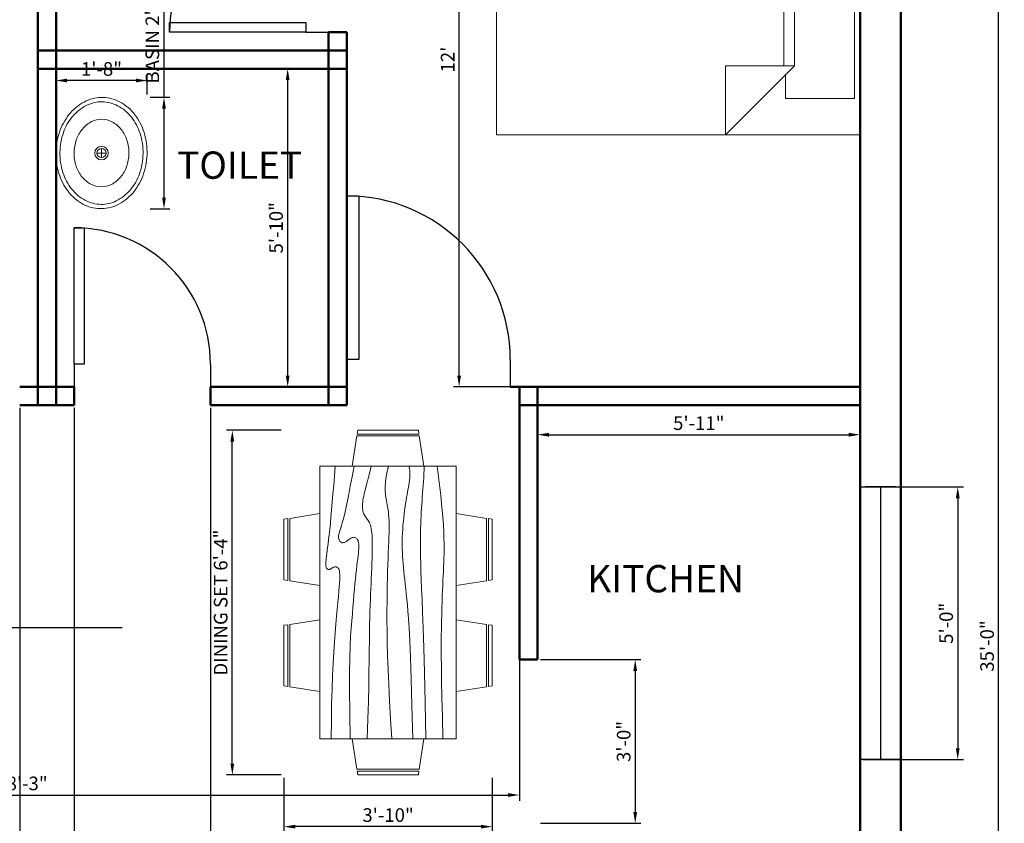
# Model space of a CAD drawing. Units: inches. Extents: x 1767 to 2185, y 3382 to 3854.
# Tile 3 of 4: x 1950 to 2167, y 3577 to 3754. Entities that reach past the tile are written whole.
import ezdxf

# ---------------------------------------------------------------- set-up
doc = ezdxf.new("R2010")
doc.units = ezdxf.units.IN
for name, color, linetype, lineweight in [('A-ANNO-DIMS', 2, 'Continuous', 18), ('A-AREA-IDEN', 7, 'Continuous', 25), ('A-DOOR', 3, 'Continuous', 25), ('A-FLOR-FIXT', 9, 'Continuous', 20), ('A-FURN', 8, 'Continuous', 18), ('A-GLAZ', 4, 'Continuous', 25), ('A-WALL', 7, 'Continuous', 50)]:
    doc.layers.add(name, color=color, linetype=linetype, lineweight=lineweight)
doc.styles.get("Standard").update_dxf_attribs({"font": 'arial.ttf'})
doc.dimstyles.new('ISO-25', dxfattribs={"dimtxt": 3, "dimasz": 2.5, "dimexe": 1.25, "dimexo": 0.625, "dimtad": 1, "dimdec": 0, "dimlunit": 3, "dimtxsty": 'Standard', "dimcen": 2.5, "dimadec": 0, "dimazin": 0, "dimtfac": 1, "dimtdec": 0, "dimtmove": 0, "dimatfit": 3, "dimfxl": 1, "dimarcsym": 0})

# ---------------------------------------------------------------- blocks, each defined once
blk = doc.blocks.new('*U2')
for p, q in [((0, 0), (0, -100)), ((600, 0), (600, -100))]:
    blk.add_line(p, q)
blk.add_lwpolyline([(0, 0), (0, 600), (43.75, 600), (43.75, 0)], close=True)
blk.add_arc((0, 0), 600, 0, 90)
blk = doc.blocks.new('*U4')
for p, q in [((0, 100), (0, 0)), ((900, 100), (900, 0)), ((0, 50), (900, 50))]:
    blk.add_line(p, q)
blk = doc.blocks.new('Dining Set - 36 x 72 in.')
for p, q in [((-22, 27.5), (-22.1562, 26.50042)), ((-5.8416, 26.5), (-22.1534, 26.5)), ((-22, 27.5), (-6, 27.5)), ((-5.8437, 26.49966), (-6, 27.5)), ((6, 27.5), (5.8438, 26.50042)), ((22.1584, 26.5), (5.8466, 26.5)), ((6, 27.5), (22, 27.5)), ((22.1563, 26.49966), (22, 27.5)), ((-22.2343, 26.00059), (-23.4847, 17.99762)), ((-22.2304, 26), (-5.7608, 26)), ((-4.5152, 17.99762), (-5.7655, 25.99926)), ((5.7657, 26.00059), (4.5153, 17.99762)), ((5.7696, 26), (22.2392, 26)), ((23.4848, 17.99762), (22.2345, 25.99926)), ((36, 18), (-36, 18)), ((-36, 18), (-36, -18)), ((36, -18), (36, 18)), ((-45.5, 8), (-44.5004, 8.15617)), ((-45.5, 8), (-45.5, -8)), ((-44.5, -8.15843), (-44.5, 8.15338)), ((-44.0006, 8.23428), (-35.9976, 9.48474)), ((-44, 8.23041), (-44, -8.23915)), ((44.0006, 8.23428), (35.9976, 9.48474)), ((44, 8.23041), (44, -8.23915)), ((44.5, -8.15843), (44.5, 8.15338)), ((45.5, 8), (44.5005, 8.15617)), ((45.5, 8), (45.5, -8)), ((-44.4997, -8.15631), (-45.5, -8)), ((-35.9976, -9.48476), (-43.9993, -8.2345)), ((35.9976, -9.48476), (43.9993, -8.2345)), ((44.4997, -8.15631), (45.5, -8)), ((-36, -18), (36, -18)), ((-22.2343, -26.0006), (-23.4847, -17.99762)), ((-4.5152, -17.99762), (-5.7655, -25.99928)), ((5.7657, -26.0006), (4.5153, -17.99762)), ((23.4848, -17.99762), (22.2345, -25.99928)), ((-22.2304, -26), (-5.7608, -26)), ((5.7696, -26), (22.2392, -26)), ((-22, -27.5), (-22.1562, -26.50044)), ((-5.8416, -26.5), (-22.1534, -26.5)), ((-22, -27.5), (-6, -27.5)), ((-5.8437, -26.49967), (-6, -27.5)), ((6, -27.5), (5.8438, -26.50044)), ((22.1584, -26.5), (5.8466, -26.5)), ((6, -27.5), (22, -27.5)), ((22.1563, -26.49967), (22, -27.5))]:
    blk.add_line(p, q)
for points in [[(-36, 15), (-31.1772, 14.97754), (-26.8079, 14.91406), (-22.8538, 14.81543), (-19.276, 14.6875), (-16.0362, 14.53613), (-13.0957, 14.36718), (-10.4159, 14.18652), (-7.9583, 14), (-5.6904, 13.81315), (-3.6035, 13.63021), (-1.6954, 13.45508), (0.0365, 13.29166), (1.5945, 13.14388), (2.9811, 13.01562), (4.1988, 12.9108), (5.25, 12.83333), (6.1393, 12.78613), (6.8802, 12.76823), (7.4883, 12.77767), (7.9792, 12.8125), (8.3685, 12.87077), (8.6719, 12.95052), (8.9049, 13.0498), (9.0833, 13.16666), (9.2205, 13.29899), (9.3216, 13.44401), (9.3895, 13.59879), (9.4271, 13.76041), (9.4373, 13.92594), (9.4232, 14.09245), (9.3875, 14.257), (9.3333, 14.41666), (9.2638, 14.56917), (9.1836, 14.71484), (9.0975, 14.85465), (9.0104, 14.98958), (8.9272, 15.1206), (8.8529, 15.2487), (8.7922, 15.37483), (8.75, 15.5), (8.7305, 15.62467), (8.7344, 15.74739), (8.7617, 15.86621), (8.8125, 15.97916), (8.8867, 16.08431), (8.9844, 16.17968), (9.1055, 16.26334), (9.25, 16.33333), (9.4189, 16.38802), (9.6172, 16.42708), (9.8506, 16.45052), (10.125, 16.45833), (10.4463, 16.45052), (10.8203, 16.42708), (11.2529, 16.38802), (11.75, 16.33333), (12.3184, 16.26318), (12.9694, 16.17838), (13.7151, 16.07991), (14.5677, 15.96875), (15.5395, 15.84586), (16.6426, 15.71224), (17.8893, 15.56884), (19.2917, 15.41666), (20.859, 15.25667), (22.5879, 15.08984), (24.4721, 14.91715), (26.5052, 14.73958), (28.6809, 14.5581), (30.9929, 14.3737), (33.4347, 14.18733), (36, 14)], [(-36, 10), (-28.9766, 10.14274), (-23.1725, 10.20442), (-18.4241, 10.19775), (-14.5677, 10.13541), (-11.4399, 10.03011), (-8.877, 9.89453), (-6.7154, 9.74137), (-4.7917, 9.58333), (-2.9698, 9.43082), (-1.2246, 9.28515), (0.4415, 9.14534), (2.026, 9.01041), (3.5266, 8.87939), (4.9408, 8.7513), (6.266, 8.62516), (7.5, 8.5), (8.6411, 8.37549), (9.6914, 8.2539), (10.6538, 8.13818), (11.5312, 8.03125), (12.3267, 7.93603), (13.043, 7.85547), (13.6831, 7.79248), (14.25, 7.75), (14.7471, 7.7303), (15.1797, 7.73307), (15.5537, 7.75732), (15.875, 7.80208), (16.1494, 7.86637), (16.3828, 7.94922), (16.5811, 8.04964), (16.75, 8.16666), (16.8944, 8.29915), (17.0143, 8.44531), (17.1089, 8.60319), (17.1771, 8.77083), (17.218, 8.94629), (17.2305, 9.1276), (17.2137, 9.31282), (17.1667, 9.5), (17.0895, 9.6875), (16.987, 9.875), (16.8649, 10.0625), (16.7292, 10.25), (16.5856, 10.4375), (16.4401, 10.625), (16.2985, 10.8125), (16.1667, 11), (16.05, 11.18733), (15.9518, 11.3737), (15.8752, 11.5581), (15.8229, 11.73958), (15.798, 11.91715), (15.8034, 12.08984), (15.842, 12.25667), (15.9167, 12.41666), (16.0295, 12.56836), (16.1784, 12.70833), (16.3605, 12.83268), (16.5729, 12.9375), (16.8127, 13.01888), (17.0768, 13.07291), (17.3625, 13.0957), (17.6667, 13.08333), (17.9894, 13.03312), (18.3418, 12.94726), (18.7382, 12.82918), (19.1927, 12.68229), (19.7195, 12.51001), (20.3327, 12.31575), (21.0465, 12.10294), (21.875, 11.875), (22.8357, 11.63354), (23.959, 11.37304), (25.2786, 11.08618), (26.8282, 10.76562), (28.6414, 10.40405), (30.752, 9.99414), (33.1936, 9.52856), (36, 9)], [(-36, 5.5), (-30.7157, 5.3348), (-26.069, 5.20963), (-21.9946, 5.11767), (-18.4271, 5.05208), (-15.3009, 5.00602), (-12.5508, 4.97265), (-10.1112, 4.94515), (-7.9167, 4.91666), (-5.909, 4.88167), (-4.0586, 4.83984), (-2.3429, 4.79215), (-0.7396, 4.73958), (0.7739, 4.6831), (2.22, 4.6237), (3.6213, 4.56233), (5, 4.5), (6.373, 4.43782), (7.7344, 4.3776), (9.0723, 4.32129), (10.375, 4.27083), (11.6309, 4.22819), (12.8281, 4.19531), (13.9551, 4.17415), (15, 4.16666), (15.954, 4.17448), (16.819, 4.19791), (17.6001, 4.23698), (18.3021, 4.29166), (18.9299, 4.36198), (19.4883, 4.44791), (19.9823, 4.54948), (20.4167, 4.66666), (20.7969, 4.79899), (21.1302, 4.94401), (21.4245, 5.09879), (21.6875, 5.26041), (21.9271, 5.42594), (22.1511, 5.59245), (22.3672, 5.757), (22.5834, 5.91666), (22.8065, 6.06868), (23.0404, 6.21093), (23.2879, 6.34147), (23.5521, 6.45833), (23.8358, 6.55957), (24.142, 6.64323), (24.4735, 6.70735), (24.8334, 6.75), (25.2235, 6.76969), (25.642, 6.76692), (26.0858, 6.74267), (26.5521, 6.69791), (27.0379, 6.63362), (27.5404, 6.55078), (28.0565, 6.45036), (28.5834, 6.33333), (29.1242, 6.19987), (29.7071, 6.04687), (30.3661, 5.87044), (31.1354, 5.66666), (32.0493, 5.43164), (33.142, 5.16146), (34.4475, 4.85221), (36, 4.5)], [(-36, -1), (-30.7915, -0.6591), (-26.0195, -0.38216), (-21.6519, -0.16284), (-17.6563, 0.00521), (-14.0005, 0.12833), (-10.6523, 0.21289), (-7.5796, 0.26522), (-4.75, 0.29166), (-2.134, 0.29793), (0.2878, 0.28711), (2.5317, 0.26163), (4.6146, 0.22396), (6.5529, 0.17651), (8.3633, 0.12174), (10.0623, 0.06209), (11.6667, 0), (13.1899, -0.06201), (14.6341, -0.1211), (15.9982, -0.17432), (17.2813, -0.21875), (18.4823, -0.25147), (19.6003, -0.26953), (20.6343, -0.27002), (21.5834, -0.25), (22.4481, -0.20768), (23.2357, -0.14584), (23.9549, -0.06836), (24.6146, 0.02083), (25.2235, 0.11784), (25.7904, 0.21875), (26.3241, 0.31966), (26.8334, 0.41666), (27.3265, 0.50618), (27.8099, 0.58593), (28.2894, 0.65397), (28.7709, 0.70833), (29.2601, 0.74707), (29.763, 0.76823), (30.2855, 0.76985), (30.8334, 0.75), (31.4088, 0.70784), (31.9994, 0.64713), (32.589, 0.57275), (33.1615, 0.48958), (33.7008, 0.4025), (34.1908, 0.3164), (34.6153, 0.23616), (34.9584, 0.16666), (35.2099, 0.11165), (35.3848, 0.07031), (35.504, 0.04069), (35.5886, 0.02083), (35.6594, 0.00879), (35.7377, 0.0026), (35.8442, 0.00032), (36, 0)], [(-36, -6.5), (-27.1843, -6.31267), (-20.084, -6.1263), (-14.469, -5.9419), (-10.1094, -5.76042), (-6.7752, -5.58285), (-4.2363, -5.41016), (-2.2629, -5.24333), (-0.625, -5.08334), (0.8708, -4.93099), (2.2715, -4.78646), (3.5872, -4.64974), (4.8281, -4.52084), (6.0046, -4.39974), (7.127, -4.28646), (8.2053, -4.18099), (9.25, -4.08334), (10.2705, -3.99382), (11.2734, -3.91407), (12.2647, -3.84603), (13.25, -3.79167), (14.2354, -3.75293), (15.2266, -3.73177), (16.2295, -3.73015), (17.25, -3.75), (18.2912, -3.79248), (19.3451, -3.85547), (20.4009, -3.93604), (21.4479, -4.03125), (22.4754, -4.13819), (23.4727, -4.25391), (24.4289, -4.37549), (25.3334, -4.5), (26.1785, -4.62492), (26.9694, -4.74935), (27.7145, -4.87281), (28.4219, -4.99479), (29.1, -5.11483), (29.7572, -5.23242), (30.4016, -5.34709), (31.0417, -5.45834), (31.6837, -5.56437), (32.3262, -5.65821), (32.9658, -5.73153), (33.599, -5.77604), (34.2224, -5.78345), (34.8327, -5.74545), (35.4264, -5.65373), (36, -5.5)], [(-36, -10), (-26.4022, -9.81299), (-18.4675, -9.62891), (-11.9839, -9.45069), (-6.7396, -9.28125), (-2.5226, -9.12354), (0.8789, -8.98047), (3.6769, -8.85498), (6.0833, -8.75), (8.2767, -8.66765), (10.3021, -8.60677), (12.1712, -8.56543), (13.8958, -8.54167), (15.4876, -8.53353), (16.9583, -8.53907), (18.3197, -8.55632), (19.5834, -8.58334), (20.7616, -8.61841), (21.8685, -8.66081), (22.9188, -8.71004), (23.9271, -8.76563), (24.9081, -8.82707), (25.8763, -8.89388), (26.8465, -8.96558), (27.8334, -9.04167), (28.8474, -9.12118), (29.8828, -9.20117), (30.93, -9.27824), (31.9792, -9.34896), (33.0205, -9.40991), (34.0443, -9.45768), (35.0407, -9.48885), (36, -9.5)], [(-36, -14.5), (-30.0881, -14.33513), (-25.0332, -14.21224), (-20.7312, -14.12647), (-17.0781, -14.07292), (-13.97, -14.04671), (-11.3027, -14.04297), (-8.9724, -14.05681), (-6.875, -14.08334), (-4.9224, -14.11833), (-3.0905, -14.16016), (-1.3709, -14.20785), (0.2448, -14.26042), (1.7647, -14.3169), (3.1973, -14.3763), (4.5507, -14.43767), (5.8333, -14.5), (7.0554, -14.5621), (8.235, -14.62175), (9.3922, -14.67652), (10.5469, -14.72396), (11.7192, -14.76164), (12.929, -14.78711), (14.1965, -14.79794), (15.5417, -14.79167), (16.9933, -14.76424), (18.6152, -14.70508), (20.4804, -14.60197), (22.6615, -14.44271), (25.2312, -14.21509), (28.2624, -13.9069), (31.8277, -13.50594), (36, -13)]]:
    blk.add_lwpolyline(points)
blk = doc.blocks.new('Sink - Oval top')
for p, q in [((-1, 0), (1, 0)), ((0, 1), (0, -1))]:
    blk.add_line(p, q)
for points in [[(-12.23, 0.39, 0.117634), (-11.46, -3.36, 0.104469), (-8.88, -6.8, 0.090016), (-5.08, -9.07, 0.08192), (-0.32, -10.02, 0.08192), (4.49, -9.38, 0.090016), (8.42, -7.36, 0.104469), (11.22, -4.09, 0.117634), (12.23, -0.39, 0.117634), (11.46, 3.36, 0.104469), (8.88, 6.8, 0.090016), (5.08, 9.07, 0.08192), (0.32, 10.02, 0.08192), (-4.49, 9.38, 0.090016), (-8.42, 7.36, 0.104469), (-11.22, 4.09, 0.117634)], [(-11.29, 0.16, 0.118622), (-10.52, -3.25, 0.104678), (-8.07, -6.36, 0.089562), (-4.54, -8.37, 0.081185), (-0.13, -9.15, 0.081185), (4.3, -8.49, 0.089562), (7.89, -6.58, 0.104678), (10.42, -3.55, 0.118622), (11.29, -0.16, 0.118622), (10.52, 3.25, 0.104678), (8.07, 6.36, 0.089562), (4.54, 8.37, 0.081185), (0.13, 9.15, 0.081185), (-4.3, 8.49, 0.089562), (-7.89, 6.58, 0.104678), (-10.42, 3.55, 0.118622)], [(-7.42, 0.08, 0.118283), (-6.91, -2.17, 0.104607), (-5.29, -4.21, 0.089718), (-2.97, -5.53, 0.081436), (-0.07, -6.04, 0.081436), (2.84, -5.59, 0.089718), (5.2, -4.33, 0.104607), (6.86, -2.32, 0.118283), (7.42, -0.08, 0.118283), (6.91, 2.17, 0.104607), (5.29, 4.21, 0.089718), (2.97, 5.53, 0.081436), (0.07, 6.04, 0.081436), (-2.84, 5.59, 0.089718), (-5.2, 4.33, 0.104607), (-6.86, 2.32, 0.118283)]]:
    blk.add_lwpolyline(points, format="xyb", close=True)
for radius in [1.5, 1]:
    blk.add_circle((0, 0), radius)
blk = doc.blocks.new('Bed - Queen')
for p, q in [((0, -80.00003), (0, 0)), ((0, 0), (59.99999, 0)), ((59.99999, 0), (59.99999, -80.00003)), ((7.99999, -1.2), (28.79998, -1.2)), ((7.99999, -14.4), (7.99999, -1.2)), ((28.79998, -1.2), (28.79998, -14.4)), ((31.19999, -1.2), (51.99999, -1.2)), ((31.19999, -14.4), (31.19999, -1.2)), ((51.99999, -1.2), (51.99999, -16.4)), ((0, -14.4), (44.8, -14.4)), ((59.99999, -29.6), (44.8, -14.4)), ((44.8, -14.4), (44.8, -29.6)), ((44.8, -16.8), (0, -16.8)), ((51.99999, -16.4), (46.79936, -16.4)), ((44.8, -29.6), (59.99999, -29.6)), ((59.99999, -80.00003), (0, -80.00003))]:
    blk.add_line(p, q)
blk = doc.blocks.new('*D13')
at = {"layer": 'A-ANNO-DIMS', "color": 0, "lineweight": -2, "transparency": 16777216}
for p, q in [((2134.53, 3817.15), (2045.65, 3817.15)), ((2046.9, 3675.65), (2046.9, 3814.65)), ((2134.53, 3673.15), (2045.65, 3673.15))]:
    blk.add_line(p, q, dxfattribs=at)
at = {"layer": 'A-ANNO-DIMS', "color": 0, "transparency": 16777216}
for points in [[(2046.48, 3814.65), (2047.32, 3814.65), (2046.9, 3817.15)], [(2046.48, 3675.65), (2047.32, 3675.65), (2046.9, 3673.15)]]:
    blk.add_solid(points, dxfattribs=at)
at = {"layer": 'Defpoints', "color": 0, "transparency": 16777216}
for p in [(2046.9, 3817.15), (2135.16, 3817.15), (2135.16, 3673.15)]:
    blk.add_point(p, dxfattribs=at)
at = {"layer": 'A-ANNO-DIMS', "color": 0, "transparency": 16777216, "insert": (2044.77, 3745.15), "char_height": 3, "attachment_point": 5, "rotation": 90}
blk.add_mtext("12'", dxfattribs=at)
blk = doc.blocks.new('*D15')
at = {"layer": 'A-ANNO-DIMS', "color": 0, "lineweight": -2, "transparency": 16777216}
for p, q in [((2017.53, 3743.15), (2007.9, 3743.15)), ((2009.15, 3740.65), (2009.15, 3675.65)), ((2017.53, 3673.15), (2007.9, 3673.15))]:
    blk.add_line(p, q, dxfattribs=at)
at = {"layer": 'A-ANNO-DIMS', "color": 0, "transparency": 16777216}
for points in [[(2008.73, 3740.65), (2009.57, 3740.65), (2009.15, 3743.15)], [(2008.73, 3675.65), (2009.57, 3675.65), (2009.15, 3673.15)]]:
    blk.add_solid(points, dxfattribs=at)
at = {"layer": 'Defpoints', "color": 0, "transparency": 16777216}
for p in [(2018.16, 3743.15), (2009.15, 3673.15), (2018.16, 3673.15)]:
    blk.add_point(p, dxfattribs=at)
at = {"layer": 'A-ANNO-DIMS', "color": 0, "transparency": 16777216, "insert": (2006.99, 3708.15), "char_height": 3, "attachment_point": 5, "rotation": 90}
blk.add_mtext('5\'-10"', dxfattribs=at)
blk = doc.blocks.new('*D16')
at = {"layer": 'A-ANNO-DIMS', "color": 0, "lineweight": -2, "transparency": 16777216}
for p, q in [((2064.16, 3668.53), (2064.16, 3661.38)), ((2135.16, 3668.53), (2135.16, 3661.38)), ((2066.66, 3662.63), (2132.66, 3662.63))]:
    blk.add_line(p, q, dxfattribs=at)
at = {"layer": 'A-ANNO-DIMS', "color": 0, "transparency": 16777216}
for points in [[(2066.66, 3663.04), (2066.66, 3662.21), (2064.16, 3662.63)], [(2132.66, 3663.04), (2132.66, 3662.21), (2135.16, 3662.63)]]:
    blk.add_solid(points, dxfattribs=at)
at = {"layer": 'Defpoints', "color": 0, "transparency": 16777216}
for p in [(2064.16, 3669.15), (2135.16, 3669.15), (2135.16, 3662.63)]:
    blk.add_point(p, dxfattribs=at)
at = {"layer": 'A-ANNO-DIMS', "color": 0, "transparency": 16777216, "insert": (2099.66, 3664.78), "char_height": 3, "attachment_point": 5}
blk.add_mtext('5\'-11"', dxfattribs=at)
blk = doc.blocks.new('*D17')
at = {"layer": 'A-ANNO-DIMS', "color": 0, "lineweight": -2, "transparency": 16777216}
for p, q in [((1841.16, 3668.53), (1841.16, 3582.12)), ((2060.16, 3668.53), (2060.16, 3582.12)), ((1843.66, 3583.37), (2057.66, 3583.37))]:
    blk.add_line(p, q, dxfattribs=at)
at = {"layer": 'A-ANNO-DIMS', "color": 0, "transparency": 16777216}
for points in [[(1843.66, 3583.79), (1843.66, 3582.96), (1841.16, 3583.37)], [(2057.66, 3583.79), (2057.66, 3582.96), (2060.16, 3583.37)]]:
    blk.add_solid(points, dxfattribs=at)
at = {"layer": 'Defpoints', "color": 0, "transparency": 16777216}
for p in [(1841.16, 3669.15), (2060.16, 3669.15), (2060.16, 3583.37)]:
    blk.add_point(p, dxfattribs=at)
at = {"layer": 'A-ANNO-DIMS', "color": 0, "transparency": 16777216, "insert": (1950.66, 3585.53), "char_height": 3, "attachment_point": 5}
blk.add_mtext('18\'-3"', dxfattribs=at)
blk = doc.blocks.new('*D31')
at = {"layer": 'A-ANNO-DIMS', "color": 0, "lineweight": -2, "transparency": 16777216}
for p, q in [((2007.72, 3663.62), (1995.72, 3663.62)), ((1996.97, 3590.29), (1996.97, 3661.12)), ((2007.72, 3587.79), (1995.72, 3587.79))]:
    blk.add_line(p, q, dxfattribs=at)
at = {"layer": 'A-ANNO-DIMS', "color": 0, "transparency": 16777216}
for points in [[(1996.55, 3661.12), (1997.38, 3661.12), (1996.97, 3663.62)], [(1996.55, 3590.29), (1997.38, 3590.29), (1996.97, 3587.79)]]:
    blk.add_solid(points, dxfattribs=at)
at = {"layer": 'Defpoints', "color": 0, "transparency": 16777216}
for p in [(1996.97, 3663.62), (2008.34, 3663.62), (2008.34, 3587.79)]:
    blk.add_point(p, dxfattribs=at)
at = {"layer": 'A-ANNO-DIMS', "color": 0, "transparency": 16777216, "insert": (1994.79, 3625.7), "char_height": 3, "attachment_point": 5, "rotation": 90}
blk.add_mtext('DINING SET 6\'-4"', dxfattribs=at)
blk = doc.blocks.new('*D32')
at = {"layer": 'A-ANNO-DIMS', "color": 0, "lineweight": -2, "transparency": 16777216}
for p, q in [((2008.34, 3587.16), (2008.34, 3575.16)), ((2054.18, 3587.16), (2054.18, 3575.16)), ((2051.68, 3576.41), (2010.84, 3576.41))]:
    blk.add_line(p, q, dxfattribs=at)
at = {"layer": 'A-ANNO-DIMS', "color": 0, "transparency": 16777216}
for points in [[(2010.84, 3576.83), (2010.84, 3576), (2008.34, 3576.41)], [(2051.68, 3576.83), (2051.68, 3576), (2054.18, 3576.41)]]:
    blk.add_solid(points, dxfattribs=at)
at = {"layer": 'Defpoints', "color": 0, "transparency": 16777216}
for p in [(2008.34, 3587.79), (2054.18, 3587.79), (2008.34, 3576.41)]:
    blk.add_point(p, dxfattribs=at)
at = {"layer": 'A-ANNO-DIMS', "color": 0, "transparency": 16777216, "insert": (2031.26, 3578.57), "char_height": 3, "attachment_point": 5}
blk.add_mtext('3\'-10"', dxfattribs=at)
blk = doc.blocks.new('*D35')
at = {"layer": 'A-ANNO-DIMS', "color": 0, "lineweight": -2, "transparency": 16777216}
for p, q in [((1981.93, 3736.86), (1981.93, 3769.19)), ((1978.87, 3736.86), (1983.18, 3736.86)), ((1981.93, 3714.81), (1981.93, 3734.36)), ((1978.87, 3712.31), (1983.18, 3712.31))]:
    blk.add_line(p, q, dxfattribs=at)
at = {"layer": 'A-ANNO-DIMS', "color": 0, "transparency": 16777216}
for points in [[(1981.51, 3734.36), (1982.34, 3734.36), (1981.93, 3736.86)], [(1981.51, 3714.81), (1982.34, 3714.81), (1981.93, 3712.31)]]:
    blk.add_solid(points, dxfattribs=at)
at = {"layer": 'Defpoints', "color": 0, "transparency": 16777216}
for p in [(1978.24, 3736.86), (1981.93, 3736.86), (1978.24, 3712.31)]:
    blk.add_point(p, dxfattribs=at)
at = {"layer": 'A-ANNO-DIMS', "color": 0, "transparency": 16777216, "insert": (1979.75, 3754.28), "char_height": 3, "attachment_point": 5, "rotation": 90}
blk.add_mtext('BASIN 2\'-0 1/2"', dxfattribs=at)
blk = doc.blocks.new('*D36')
at = {"layer": 'A-ANNO-DIMS', "color": 0, "lineweight": -2, "transparency": 16777216}
for p, q in [((1958.11, 3737.49), (1958.11, 3741.8)), ((1978.24, 3737.49), (1978.24, 3741.8)), ((1975.74, 3740.55), (1960.61, 3740.55))]:
    blk.add_line(p, q, dxfattribs=at)
at = {"layer": 'A-ANNO-DIMS', "color": 0, "transparency": 16777216}
for points in [[(1960.61, 3740.96), (1960.61, 3740.13), (1958.11, 3740.55)], [(1975.74, 3740.96), (1975.74, 3740.13), (1978.24, 3740.55)]]:
    blk.add_solid(points, dxfattribs=at)
at = {"layer": 'Defpoints', "color": 0, "transparency": 16777216}
for p in [(1958.11, 3740.55), (1958.11, 3736.86), (1978.24, 3736.86)]:
    blk.add_point(p, dxfattribs=at)
at = {"layer": 'A-ANNO-DIMS', "color": 0, "transparency": 16777216, "insert": (1968.17, 3742.7), "char_height": 3, "attachment_point": 5}
blk.add_mtext('1\'-8"', dxfattribs=at)
blk = doc.blocks.new('*D40')
at = {"layer": 'A-ANNO-DIMS', "color": 0, "lineweight": -2, "transparency": 16777216}
for p, q in [((2144.78, 3826.15), (2166.91, 3826.15)), ((2165.66, 3408.65), (2165.66, 3823.65)), ((2144.78, 3406.15), (2166.91, 3406.15))]:
    blk.add_line(p, q, dxfattribs=at)
at = {"layer": 'A-ANNO-DIMS', "color": 0, "transparency": 16777216}
for points in [[(2165.25, 3823.65), (2166.08, 3823.65), (2165.66, 3826.15)], [(2165.25, 3408.65), (2166.08, 3408.65), (2165.66, 3406.15)]]:
    blk.add_solid(points, dxfattribs=at)
at = {"layer": 'Defpoints', "color": 0, "transparency": 16777216}
for p in [(2144.16, 3826.15), (2165.66, 3826.15), (2144.16, 3406.15)]:
    blk.add_point(p, dxfattribs=at)
at = {"layer": 'A-ANNO-DIMS', "color": 0, "transparency": 16777216, "insert": (2163.51, 3616.15), "char_height": 3, "attachment_point": 5, "rotation": 90}
blk.add_mtext('35\'-0"', dxfattribs=at)
blk = doc.blocks.new('*D42')
at = {"layer": 'A-ANNO-DIMS', "color": 0, "lineweight": -2, "transparency": 16777216}
for p, q in [((1914.16, 3668.53), (1914.16, 3383.4)), ((1950.16, 3668.53), (1950.16, 3383.4)), ((1916.66, 3384.65), (1947.66, 3384.65))]:
    blk.add_line(p, q, dxfattribs=at)
at = {"layer": 'A-ANNO-DIMS', "color": 0, "transparency": 16777216}
for points in [[(1916.66, 3385.06), (1916.66, 3384.23), (1914.16, 3384.65)], [(1947.66, 3385.06), (1947.66, 3384.23), (1950.16, 3384.65)]]:
    blk.add_solid(points, dxfattribs=at)
at = {"layer": 'Defpoints', "color": 0, "transparency": 16777216}
for p in [(1914.16, 3669.15), (1950.16, 3669.15), (1950.16, 3384.65)]:
    blk.add_point(p, dxfattribs=at)
at = {"layer": 'A-ANNO-DIMS', "color": 0, "transparency": 16777216, "insert": (1932.16, 3386.8), "char_height": 3, "attachment_point": 5}
blk.add_mtext('3\'-0"', dxfattribs=at)
blk = doc.blocks.new('*D43')
at = {"layer": 'A-ANNO-DIMS', "color": 0, "lineweight": -2, "transparency": 16777216}
for p, q in [((1962.16, 3668.53), (1962.16, 3383.4)), ((1992.16, 3668.53), (1992.16, 3383.4)), ((1964.66, 3384.65), (1989.66, 3384.65))]:
    blk.add_line(p, q, dxfattribs=at)
at = {"layer": 'A-ANNO-DIMS', "color": 0, "transparency": 16777216}
for points in [[(1964.66, 3385.06), (1964.66, 3384.23), (1962.16, 3384.65)], [(1989.66, 3385.06), (1989.66, 3384.23), (1992.16, 3384.65)]]:
    blk.add_solid(points, dxfattribs=at)
at = {"layer": 'Defpoints', "color": 0, "transparency": 16777216}
for p in [(1962.16, 3669.15), (1992.16, 3669.15), (1992.16, 3384.65)]:
    blk.add_point(p, dxfattribs=at)
at = {"layer": 'A-ANNO-DIMS', "color": 0, "transparency": 16777216, "insert": (1977.16, 3386.8), "char_height": 3, "attachment_point": 5}
blk.add_mtext('2\'-6"', dxfattribs=at)
blk = doc.blocks.new('*D45')
at = {"layer": 'A-ANNO-DIMS', "color": 0, "lineweight": -2, "transparency": 16777216}
for p, q in [((2135.78, 3651.15), (2157.91, 3651.15)), ((2156.66, 3648.65), (2156.66, 3593.65)), ((2135.78, 3591.15), (2157.91, 3591.15))]:
    blk.add_line(p, q, dxfattribs=at)
at = {"layer": 'A-ANNO-DIMS', "color": 0, "transparency": 16777216}
for points in [[(2156.25, 3648.65), (2157.08, 3648.65), (2156.66, 3651.15)], [(2156.25, 3593.65), (2157.08, 3593.65), (2156.66, 3591.15)]]:
    blk.add_solid(points, dxfattribs=at)
at = {"layer": 'Defpoints', "color": 0, "transparency": 16777216}
for p in [(2135.16, 3651.15), (2135.16, 3591.15), (2156.66, 3591.15)]:
    blk.add_point(p, dxfattribs=at)
at = {"layer": 'A-ANNO-DIMS', "color": 0, "transparency": 16777216, "insert": (2154.51, 3621.15), "char_height": 3, "attachment_point": 5, "rotation": 90}
blk.add_mtext('5\'-0"', dxfattribs=at)
blk = doc.blocks.new('*D48')
at = {"layer": 'A-ANNO-DIMS', "color": 0, "lineweight": -2, "transparency": 16777216}
for p, q in [((2064.78, 3613.15), (2086.91, 3613.15)), ((2085.66, 3610.65), (2085.66, 3579.65)), ((2064.78, 3577.15), (2086.91, 3577.15))]:
    blk.add_line(p, q, dxfattribs=at)
at = {"layer": 'A-ANNO-DIMS', "color": 0, "transparency": 16777216}
for points in [[(2085.25, 3610.65), (2086.08, 3610.65), (2085.66, 3613.15)], [(2085.25, 3579.65), (2086.08, 3579.65), (2085.66, 3577.15)]]:
    blk.add_solid(points, dxfattribs=at)
at = {"layer": 'Defpoints', "color": 0, "transparency": 16777216}
for p in [(2064.16, 3613.15), (2064.16, 3577.15), (2085.66, 3577.15)]:
    blk.add_point(p, dxfattribs=at)
at = {"layer": 'A-ANNO-DIMS', "color": 0, "transparency": 16777216, "insert": (2083.51, 3595.15), "char_height": 3, "attachment_point": 5, "rotation": 90}
blk.add_mtext('3\'-0"', dxfattribs=at)
blk = doc.blocks.new('*D51')
at = {"layer": 'A-ANNO-DIMS', "color": 0, "lineweight": -2, "transparency": 16777216}
for p, q in [((1771.61, 3620.13), (1849.04, 3620.13)), ((1972.74, 3620.13), (1851.54, 3620.13))]:
    blk.add_line(p, q, dxfattribs=at)
at = {"layer": 'A-ANNO-DIMS', "color": 0, "transparency": 16777216}
blk.add_solid([(1849.04, 3620.54), (1849.04, 3619.71), (1851.54, 3620.13)], dxfattribs=at)
at = {"layer": 'Defpoints', "color": 0, "transparency": 16777216}
for p in [(1851.54, 3620.13), (1972.74, 3620.13)]:
    blk.add_point(p, dxfattribs=at)
at = {"layer": 'A-ANNO-DIMS', "color": 0, "transparency": 16777216, "insert": (1778.83, 3622.28), "char_height": 3, "attachment_point": 5, "rotation": 359.9999}
blk.add_mtext('R10\'-1"', dxfattribs=at)
blk = doc.blocks.new('*D52')
at = {"layer": 'A-ANNO-DIMS', "color": 0, "lineweight": -2, "transparency": 16777216}
for p, q in [((1767.45, 3620.13), (1843.04, 3620.13)), ((1959.79, 3620.13), (1845.54, 3620.13))]:
    blk.add_line(p, q, dxfattribs=at)
at = {"layer": 'A-ANNO-DIMS', "color": 0, "transparency": 16777216}
blk.add_solid([(1843.04, 3620.54), (1843.04, 3619.71), (1845.54, 3620.13)], dxfattribs=at)
at = {"layer": 'Defpoints', "color": 0, "transparency": 16777216}
for p in [(1845.54, 3620.13), (1959.79, 3620.13)]:
    blk.add_point(p, dxfattribs=at)
at = {"layer": 'A-ANNO-DIMS', "color": 0, "transparency": 16777216, "insert": (1776.99, 3622.3), "char_height": 3, "attachment_point": 5, "rotation": 359.9999}
blk.add_mtext('R9\'-6 1/2"', dxfattribs=at)

msp = doc.modelspace()

# ---------------------------------------------------------------- linework, layer by layer
at = {"layer": 'A-GLAZ'}
for p, q in [((2135.16, 3651.15), (2144.16, 3651.15)), ((2144.16, 3651.15), (2144.16, 3591.15)), ((2144.16, 3591.15), (2135.16, 3591.15))]:
    msp.add_line(p, q, dxfattribs=at)
at = {"layer": 'A-WALL'}
for p, q in [((2144.16, 3826.15), (2144.16, 3406.15)), ((1954.16, 3669.15), (1954.16, 3817.15)), ((1958.16, 3669.15), (1958.16, 3817.15)), ((2135.16, 3817.15), (2135.16, 3415.15)), ((2022.16, 3751.15), (2018.16, 3751.15)), ((2018.16, 3751.15), (2018.16, 3669.15)), ((2022.16, 3751.15), (2022.16, 3669.15)), ((1954.16, 3747.15), (2022.16, 3747.15)), ((1954.16, 3743.15), (2022.16, 3743.15)), ((1950.16, 3673.15), (1962.16, 3673.15)), ((1962.16, 3669.15), (1962.16, 3673.15)), ((1992.16, 3673.15), (1992.16, 3669.15)), ((1992.16, 3673.15), (2022.16, 3673.15)), ((2058.16, 3673.15), (2135.16, 3673.15)), ((2060.16, 3673.15), (2060.16, 3613.15)), ((2064.16, 3673.15), (2064.16, 3613.15)), ((1950.16, 3669.15), (1962.16, 3669.15)), ((1992.16, 3669.15), (2022.16, 3669.15)), ((2060.16, 3669.15), (2135.16, 3669.15)), ((2064.16, 3613.15), (2060.16, 3613.15))]:
    msp.add_line(p, q, dxfattribs=at)

# ---------------------------------------------------------------- block references
at = {"layer": 'A-DOOR', "xscale": 0.0500000000000001, "yscale": 0.0500000000000001, "zscale": 0.0500000000000001, "rotation": 90}
msp.add_blockref('*U2', (2013.16, 3751.15), dxfattribs=at)
at = {"layer": 'A-DOOR'}
for p, xscale, yscale, zscale in [((2022.16, 3679.15), 0.0599999999999998, 0.0599999999999998, 0.0599999999999998), ((1962.16, 3678.15), 0.0500000000000001, 0.0500000000000001, 0.0500000000000001)]:
    msp.add_blockref('*U2', p, dxfattribs=dict(at, xscale=xscale, yscale=yscale, zscale=zscale))
at = {"layer": 'A-FLOR-FIXT', "rotation": 90}
msp.add_blockref('Sink - Oval top', (1968.17, 3724.59), dxfattribs=at)
at = {"layer": 'A-FURN', "rotation": 269.9999999999998}
msp.add_blockref('Bed - Queen', (2135.16, 3788.57), dxfattribs=at)
at = {"layer": 'A-FURN', "xscale": 0.8333333333333385, "yscale": 0.8333333333333385, "zscale": 0.8333333333333385, "rotation": 90}
msp.add_blockref('Dining Set - 36 x 72 in.', (2031.26, 3625.7), dxfattribs=at)
at = {"layer": 'A-GLAZ', "xscale": 0.0666666666666669, "yscale": 0.0666666666666669, "zscale": 0.0666666666666669, "rotation": 270}
msp.add_blockref('*U4', (2136.33, 3651.15), dxfattribs=at)

# ---------------------------------------------------------------- texts
at = {"layer": 'A-AREA-IDEN'}
for s, p in [('TOILET', (1984.8, 3718.93)), ('KITCHEN', (2075.09, 3627.96))]:
    msp.add_text(s, height=6, dxfattribs=at).set_placement(p)

# ---------------------------------------------------------------- dimensions: what is measured, and where the dimension line sits
at = {"layer": 'A-ANNO-DIMS'}
for base, p1, p2, angle, override, picture, middle in [((2165.66, 3826.15), (2144.16, 3406.15), (2144.16, 3826.15), 90, {"dimdec": 1, "dimlfac": 1, "dimrnd": 0, "dimzin": 1, "dimdsep": 46, "dimlunit": 4, "dimfrac": 2}, '*D40', (2163.51, 3616.15)), ((2046.9, 3817.15), (2135.16, 3673.15), (2135.16, 3817.15), 90, {"dimclrd": 0, "dimclre": 0, "dimclrt": 0}, '*D13', (2044.77, 3745.15)), ((1958.11, 3740.55), (1978.24, 3736.86), (1958.11, 3736.86), 180, {"dimdec": 1, "dimlfac": 1, "dimrnd": 0, "dimzin": 1, "dimdsep": 46, "dimlunit": 4, "dimfrac": 2}, '*D36', (1968.17, 3742.7)), ((2009.15, 3673.15), (2018.16, 3743.15), (2018.16, 3673.15), 90, {"dimclrd": 0, "dimclre": 0, "dimclrt": 0}, '*D15', (2006.99, 3708.15)), ((2156.66, 3591.15), (2135.16, 3651.15), (2135.16, 3591.15), 270, {"dimdec": 1, "dimlfac": 1, "dimrnd": 0, "dimzin": 1, "dimdsep": 46, "dimlunit": 4, "dimfrac": 2}, '*D45', (2154.51, 3621.15)), ((2085.66, 3577.15), (2064.16, 3613.15), (2064.16, 3577.15), 270, {"dimdec": 1, "dimlfac": 1, "dimrnd": 0, "dimzin": 1, "dimdsep": 46, "dimlunit": 4, "dimfrac": 2}, '*D48', (2083.51, 3595.15)), ((2008.34, 3576.41), (2054.18, 3587.79), (2008.34, 3587.79), 180, {"dimdec": 1, "dimlfac": 1, "dimrnd": 0, "dimzin": 1, "dimdsep": 46, "dimlunit": 4, "dimfrac": 2}, '*D32', (2031.26, 3578.57))]:
    dim = msp.add_linear_dim(base=base, p1=p1, p2=p2, angle=angle, dimstyle='ISO-25', override=override, dxfattribs=at)
    dim.commit()
    dim.dimension.update_dxf_attribs({"geometry": picture, "text_midpoint": middle})
for base, p1, p2, text, picture, middle in [((1981.9259, 3736.8648), (1978.2433, 3712.3139), (1978.2433, 3736.8648), 'BASIN <>', '*D35', (1979.7498, 3754.2766)), ((1996.97, 3663.62), (2008.34, 3587.79), (2008.34, 3663.62), 'DINING SET <>', '*D31', (1994.79, 3625.7))]:
    dim = msp.add_linear_dim(base=base, p1=p1, p2=p2, angle=90, text=text, dimstyle='ISO-25', override={"dimdec": 1, "dimlfac": 1, "dimrnd": 0, "dimzin": 1, "dimdsep": 46, "dimlunit": 4, "dimfrac": 2}, dxfattribs=at)
    dim.commit()
    dim.dimension.update_dxf_attribs({"geometry": picture, "text_midpoint": middle})
for base, p1, p2, override, picture, middle in [((2060.16, 3583.37), (1841.16, 3669.15), (2060.16, 3669.15), {"dimclrd": 0, "dimclre": 0, "dimclrt": 0}, '*D17', (1950.66, 3585.53)), ((1950.16, 3384.65), (1914.16, 3669.15), (1950.16, 3669.15), {"dimdec": 1, "dimlfac": 1, "dimrnd": 0, "dimzin": 1, "dimdsep": 46, "dimlunit": 4, "dimfrac": 2}, '*D42', (1932.16, 3386.8)), ((1992.16, 3384.65), (1962.16, 3669.15), (1992.16, 3669.15), {"dimdec": 1, "dimlfac": 1, "dimrnd": 0, "dimzin": 1, "dimdsep": 46, "dimlunit": 4, "dimfrac": 2}, '*D43', (1977.16, 3386.8)), ((2135.16, 3662.63), (2064.16, 3669.15), (2135.16, 3669.15), {"dimclrd": 0, "dimclre": 0, "dimclrt": 0}, '*D16', (2099.66, 3664.78))]:
    dim = msp.add_linear_dim(base=base, p1=p1, p2=p2, dimstyle='ISO-25', override=override, dxfattribs=at)
    dim.commit()
    dim.dimension.update_dxf_attribs({"geometry": picture, "text_midpoint": middle})
for center, mpoint, picture, middle in [((1959.793426, 3620.126703), (1845.543426, 3620.127), '*D52', (1776.993426, 3620.1271782)), ((1972.74, 3620.13), (1851.54, 3620.13), '*D51', (1778.83, 3620.13))]:
    dim = msp.add_radius_dim(center=center, mpoint=mpoint, dimstyle='ISO-25', override={"dimdec": 1, "dimlfac": 1, "dimrnd": 0, "dimzin": 1, "dimdsep": 46, "dimlunit": 4, "dimfrac": 2}, dxfattribs=at)
    dim.commit()
    dim.dimension.update_dxf_attribs({"geometry": picture, "text_midpoint": middle, "dimtype": 164})

doc.saveas('drawing.dxf')
